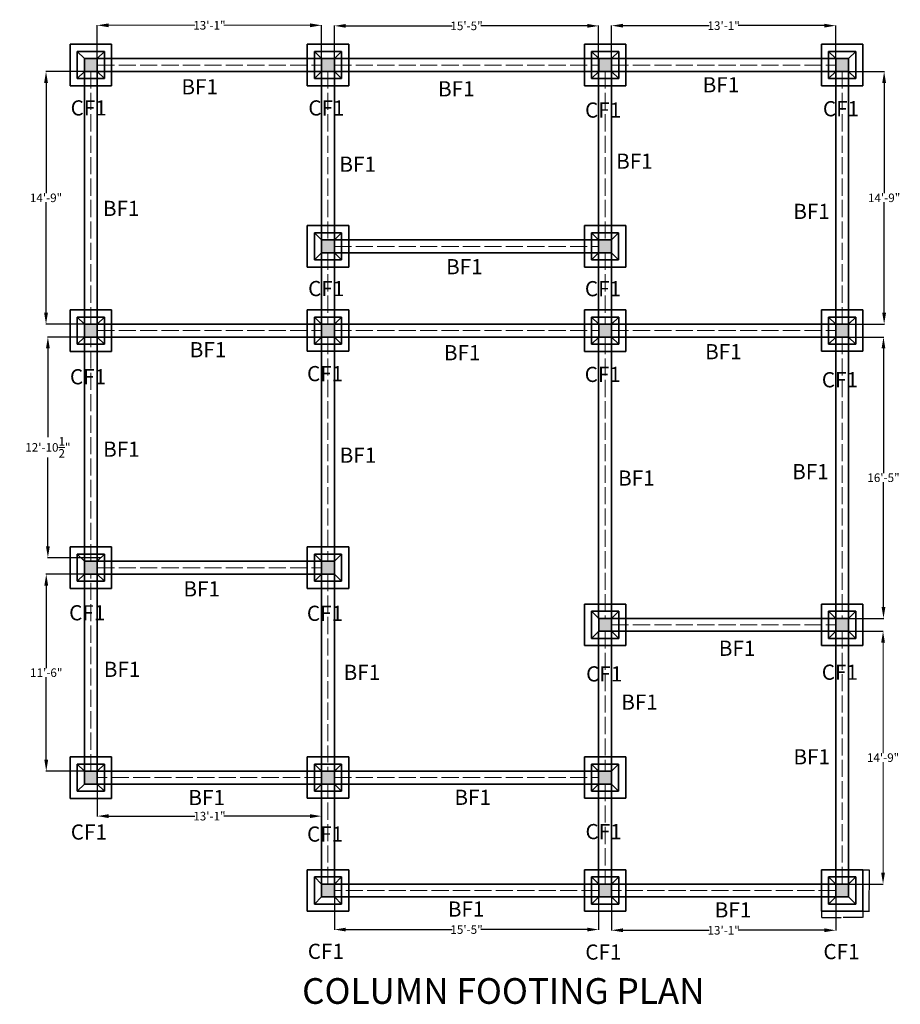
# Model space of a CAD drawing. Units: inches. Extents: x -105 to 1196, y -792 to 119.
# Tile 23 of 23: x 579 to 1196, y -592 to 97. Entities that reach past the tile are written whole.
import ezdxf

# ---------------------------------------------------------------- set-up
doc = ezdxf.new("R2010")
doc.units = ezdxf.units.IN
doc.header["$MEASUREMENT"] = 0
doc.linetypes.add('ACAD_ISO02W100', pattern=[15, 12, -3])
for name, color, linetype, lineweight in [('A-ANNO-DIMS', 2, 'Continuous', 18), ('A-ANNO-TEXT', 7, 'Continuous', 25), ('S-BEAM', 2, 'Continuous', 35), ('S-COLS', 7, 'Continuous', 35), ('S-FNDN', 7, 'Continuous', 35), ('S-GRID', 1, 'ACAD_ISO02W100', 18)]:
    doc.layers.add(name, color=color, linetype=linetype, lineweight=lineweight)
doc.styles.get("Standard").update_dxf_attribs({"font": 'arial.ttf'})
doc.dimstyles.get("Standard").update_dxf_attribs({"dimtxt": 0.18, "dimasz": 0.18, "dimexe": 0.18, "dimexo": 0.0625, "dimgap": 0.09, "dimtad": 0, "dimtih": 1, "dimtoh": 1, "dimdec": 1, "dimzin": 0, "dimdsep": 46, "dimlunit": 4, "dimtxsty": 'Standard', "dimcen": 0.09, "dimadec": 0, "dimazin": 0, "dimtfac": 1, "dimtdec": 1, "dimtofl": 0, "dimtmove": 0, "dimatfit": 3, "dimfxl": 1, "dimtolj": 1, "dimtzin": 0, "dimarcsym": 0})

# ---------------------------------------------------------------- blocks, each defined once
blk = doc.blocks.new('*D40')
at = {"layer": 'A-ANNO-DIMS', "color": 0, "lineweight": -2, "transparency": 16777216}
for p, q in [((799.59, -508.29), (799.59, -540.3)), ((984.59, -508.29), (984.59, -540.3)), ((807.59, -540.12), (881.98, -540.12)), ((976.59, -540.12), (902.21, -540.12))]:
    blk.add_line(p, q, dxfattribs=at)
at = {"layer": 'A-ANNO-DIMS', "color": 0, "transparency": 16777216}
for points in [[(807.59, -538.79), (807.59, -541.46), (799.59, -540.12)], [(976.59, -538.79), (976.59, -541.46), (984.59, -540.12)]]:
    blk.add_solid(points, dxfattribs=at)
at = {"layer": 'Defpoints', "color": 0, "transparency": 16777216}
for p in [(799.59, -508.23), (984.59, -508.23), (984.59, -540.12)]:
    blk.add_point(p, dxfattribs=at)
at = {"layer": 'A-ANNO-DIMS', "color": 0, "transparency": 16777216, "insert": (892.09, -540.12), "char_height": 6, "attachment_point": 5}
blk.add_mtext('\\A1;15\'-5"', dxfattribs=at)
blk = doc.blocks.new('*D41')
at = {"layer": 'A-ANNO-DIMS', "color": 0, "lineweight": -2, "transparency": 16777216}
for p, q in [((993.59, -508.29), (993.59, -540.79)), ((1150.59, -508.29), (1150.59, -540.79)), ((1001.59, -540.61), (1061.98, -540.61)), ((1142.59, -540.61), (1082.21, -540.61))]:
    blk.add_line(p, q, dxfattribs=at)
at = {"layer": 'A-ANNO-DIMS', "color": 0, "transparency": 16777216}
for points in [[(1001.59, -539.27), (1001.59, -541.94), (993.59, -540.61)], [(1142.59, -539.27), (1142.59, -541.94), (1150.59, -540.61)]]:
    blk.add_solid(points, dxfattribs=at)
at = {"layer": 'Defpoints', "color": 0, "transparency": 16777216}
for p in [(993.59, -508.23), (1150.59, -508.23), (1150.59, -540.61)]:
    blk.add_point(p, dxfattribs=at)
at = {"layer": 'A-ANNO-DIMS', "color": 0, "transparency": 16777216, "insert": (1072.09, -540.61), "char_height": 6, "attachment_point": 5}
blk.add_mtext('\\A1;13\'-1"', dxfattribs=at)
blk = doc.blocks.new('*D42')
at = {"layer": 'A-ANNO-DIMS', "color": 0, "lineweight": -2, "transparency": 16777216}
for p, q in [((633.59, -429.29), (633.59, -460.86)), ((790.59, -429.29), (790.59, -460.86)), ((641.59, -460.68), (701.98, -460.68)), ((782.59, -460.68), (722.21, -460.68))]:
    blk.add_line(p, q, dxfattribs=at)
at = {"layer": 'A-ANNO-DIMS', "color": 0, "transparency": 16777216}
for points in [[(641.59, -459.35), (641.59, -462.02), (633.59, -460.68)], [(782.59, -459.35), (782.59, -462.02), (790.59, -460.68)]]:
    blk.add_solid(points, dxfattribs=at)
at = {"layer": 'Defpoints', "color": 0, "transparency": 16777216}
for p in [(633.59, -429.23), (790.59, -429.23), (790.59, -460.68)]:
    blk.add_point(p, dxfattribs=at)
at = {"layer": 'A-ANNO-DIMS', "color": 0, "transparency": 16777216, "insert": (712.09, -460.68), "char_height": 6, "attachment_point": 5}
blk.add_mtext('\\A1;13\'-1"', dxfattribs=at)
blk = doc.blocks.new('*D43')
at = {"layer": 'A-ANNO-DIMS', "color": 0, "lineweight": -2, "transparency": 16777216}
for p, q in [((1150.66, -331.23), (1183.88, -331.23)), ((1150.66, -508.23), (1183.88, -508.23))]:
    blk.add_line(p, q, dxfattribs=at)
at = {"layer": 'A-ANNO-DIMS', "color": 0, "lineweight": 9, "transparency": 16777216}
for p, q in [((1183.7, -339.23), (1183.7, -416.57)), ((1183.7, -500.23), (1183.7, -422.88))]:
    blk.add_line(p, q, dxfattribs=at)
at = {"layer": 'A-ANNO-DIMS', "color": 0, "transparency": 16777216}
for points in [[(1182.36, -339.23), (1185.03, -339.23), (1183.7, -331.23)], [(1182.36, -500.23), (1185.03, -500.23), (1183.7, -508.23)]]:
    blk.add_solid(points, dxfattribs=at)
at = {"layer": 'Defpoints', "color": 0, "transparency": 16777216}
for p in [(1150.59, -331.23), (1183.7, -331.23), (1150.59, -508.23)]:
    blk.add_point(p, dxfattribs=at)
at = {"layer": 'A-ANNO-DIMS', "color": 0, "transparency": 16777216, "insert": (1183.7, -419.73), "char_height": 6, "attachment_point": 5}
blk.add_mtext('\\A1;14\'-9"', dxfattribs=at)
blk = doc.blocks.new('*D44')
at = {"layer": 'A-ANNO-DIMS', "color": 0, "lineweight": -2, "transparency": 16777216}
for p, q in [((1150.66, -125.23), (1184.17, -125.23)), ((1183.99, -133.23), (1183.99, -220.57)), ((1183.99, -314.23), (1183.99, -226.88)), ((1150.66, -322.23), (1184.17, -322.23))]:
    blk.add_line(p, q, dxfattribs=at)
at = {"layer": 'A-ANNO-DIMS', "color": 0, "transparency": 16777216}
for points in [[(1182.66, -133.23), (1185.32, -133.23), (1183.99, -125.23)], [(1182.66, -314.23), (1185.32, -314.23), (1183.99, -322.23)]]:
    blk.add_solid(points, dxfattribs=at)
at = {"layer": 'Defpoints', "color": 0, "transparency": 16777216}
for p in [(1150.59, -125.23), (1183.99, -125.23), (1150.59, -322.23)]:
    blk.add_point(p, dxfattribs=at)
at = {"layer": 'A-ANNO-DIMS', "color": 0, "transparency": 16777216, "insert": (1183.99, -223.73), "char_height": 6, "attachment_point": 5}
blk.add_mtext('\\A1;16\'-5"', dxfattribs=at)
blk = doc.blocks.new('*D45')
at = {"layer": 'A-ANNO-DIMS', "color": 0, "lineweight": -2, "transparency": 16777216}
for p, q in [((1150.66, 60.77), (1184.63, 60.77)), ((1184.45, 52.77), (1184.45, -24.57)), ((1184.45, -108.23), (1184.45, -30.88)), ((1150.66, -116.23), (1184.63, -116.23))]:
    blk.add_line(p, q, dxfattribs=at)
at = {"layer": 'A-ANNO-DIMS', "color": 0, "transparency": 16777216}
for points in [[(1183.12, 52.77), (1185.79, 52.77), (1184.45, 60.77)], [(1183.12, -108.23), (1185.79, -108.23), (1184.45, -116.23)]]:
    blk.add_solid(points, dxfattribs=at)
at = {"layer": 'Defpoints', "color": 0, "transparency": 16777216}
for p in [(1150.59, 60.77), (1184.45, 60.77), (1150.59, -116.23)]:
    blk.add_point(p, dxfattribs=at)
at = {"layer": 'A-ANNO-DIMS', "color": 0, "transparency": 16777216, "insert": (1184.45, -27.73), "char_height": 6, "attachment_point": 5}
blk.add_mtext('\\A1;14\'-9"', dxfattribs=at)
blk = doc.blocks.new('*D46')
at = {"layer": 'A-ANNO-DIMS', "color": 0, "lineweight": -2, "transparency": 16777216}
for p, q in [((993.59, 60.84), (993.59, 93)), ((1001.59, 92.82), (1061.98, 92.82)), ((1142.59, 92.82), (1082.21, 92.82)), ((1150.59, 60.84), (1150.59, 93))]:
    blk.add_line(p, q, dxfattribs=at)
at = {"layer": 'A-ANNO-DIMS', "color": 0, "transparency": 16777216}
for points in [[(1001.59, 94.15), (1001.59, 91.49), (993.59, 92.82)], [(1142.59, 94.15), (1142.59, 91.49), (1150.59, 92.82)]]:
    blk.add_solid(points, dxfattribs=at)
at = {"layer": 'Defpoints', "color": 0, "transparency": 16777216}
for p in [(1150.59, 92.82), (993.59, 60.77), (1150.59, 60.77)]:
    blk.add_point(p, dxfattribs=at)
at = {"layer": 'A-ANNO-DIMS', "color": 0, "transparency": 16777216, "insert": (1072.09, 92.82), "char_height": 6, "attachment_point": 5}
blk.add_mtext('\\A1;13\'-1"', dxfattribs=at)
blk = doc.blocks.new('*D47')
at = {"layer": 'A-ANNO-DIMS', "color": 0, "lineweight": -2, "transparency": 16777216}
for p, q in [((799.59, 60.84), (799.59, 92.86)), ((807.59, 92.68), (881.98, 92.68)), ((976.59, 92.68), (902.21, 92.68)), ((984.59, 60.84), (984.59, 92.86))]:
    blk.add_line(p, q, dxfattribs=at)
at = {"layer": 'A-ANNO-DIMS', "color": 0, "transparency": 16777216}
for points in [[(807.59, 94.02), (807.59, 91.35), (799.59, 92.68)], [(976.59, 94.02), (976.59, 91.35), (984.59, 92.68)]]:
    blk.add_solid(points, dxfattribs=at)
at = {"layer": 'Defpoints', "color": 0, "transparency": 16777216}
for p in [(984.59, 92.68), (799.59, 60.77), (984.59, 60.77)]:
    blk.add_point(p, dxfattribs=at)
at = {"layer": 'A-ANNO-DIMS', "color": 0, "transparency": 16777216, "insert": (892.09, 92.68), "char_height": 6, "attachment_point": 5}
blk.add_mtext('\\A1;15\'-5"', dxfattribs=at)
blk = doc.blocks.new('*D48')
at = {"layer": 'A-ANNO-DIMS', "color": 0, "lineweight": -2, "transparency": 16777216}
for p, q in [((633.59, 60.84), (633.59, 93.25)), ((790.59, 60.84), (790.59, 93.25))]:
    blk.add_line(p, q, dxfattribs=at)
at = {"layer": 'A-ANNO-DIMS', "color": 0, "lineweight": 5, "transparency": 16777216}
for p, q in [((641.59, 93.07), (701.98, 93.07)), ((782.59, 93.07), (722.21, 93.07))]:
    blk.add_line(p, q, dxfattribs=at)
at = {"layer": 'A-ANNO-DIMS', "color": 0, "transparency": 16777216}
for points in [[(641.59, 94.4), (641.59, 91.73), (633.59, 93.07)], [(782.59, 94.4), (782.59, 91.73), (790.59, 93.07)]]:
    blk.add_solid(points, dxfattribs=at)
at = {"layer": 'Defpoints', "color": 0, "transparency": 16777216}
for p in [(790.59, 93.07), (633.59, 60.77), (790.59, 60.77)]:
    blk.add_point(p, dxfattribs=at)
at = {"layer": 'A-ANNO-DIMS', "color": 0, "transparency": 16777216, "insert": (712.09, 93.07), "char_height": 6, "attachment_point": 5}
blk.add_mtext('\\A1;13\'-1"', dxfattribs=at)
blk = doc.blocks.new('*D49')
at = {"layer": 'A-ANNO-DIMS', "color": 0, "lineweight": -2, "transparency": 16777216}
for p, q in [((633.53, 60.77), (597.53, 60.77)), ((597.71, 52.77), (597.71, -24.57)), ((597.71, -108.23), (597.71, -30.88)), ((633.53, -116.23), (597.53, -116.23))]:
    blk.add_line(p, q, dxfattribs=at)
at = {"layer": 'A-ANNO-DIMS', "color": 0, "transparency": 16777216}
for points in [[(596.38, 52.77), (599.04, 52.77), (597.71, 60.77)], [(596.38, -108.23), (599.04, -108.23), (597.71, -116.23)]]:
    blk.add_solid(points, dxfattribs=at)
at = {"layer": 'Defpoints', "color": 0, "transparency": 16777216}
for p in [(633.59, 60.77), (597.71, -116.23), (633.59, -116.23)]:
    blk.add_point(p, dxfattribs=at)
at = {"layer": 'A-ANNO-DIMS', "color": 0, "transparency": 16777216, "insert": (597.71, -27.73), "char_height": 6, "attachment_point": 5}
blk.add_mtext('\\A1;14\'-9"', dxfattribs=at)
blk = doc.blocks.new('*D50')
at = {"layer": 'A-ANNO-DIMS', "color": 0, "lineweight": -2, "transparency": 16777216}
for p, q in [((633.53, -125.23), (598.82, -125.23)), ((599, -133.23), (599, -195.31)), ((599, -271.73), (599, -209.64)), ((636.03, -279.73), (598.82, -279.73))]:
    blk.add_line(p, q, dxfattribs=at)
at = {"layer": 'A-ANNO-DIMS', "color": 0, "transparency": 16777216}
for points in [[(597.67, -133.23), (600.33, -133.23), (599, -125.23)], [(597.67, -271.73), (600.33, -271.73), (599, -279.73)]]:
    blk.add_solid(points, dxfattribs=at)
at = {"layer": 'Defpoints', "color": 0, "transparency": 16777216}
for p in [(633.59, -125.23), (599, -279.73), (636.09, -279.73)]:
    blk.add_point(p, dxfattribs=at)
at = {"layer": 'A-ANNO-DIMS', "color": 0, "transparency": 16777216, "insert": (599, -202.48), "char_height": 6, "attachment_point": 5}
blk.add_mtext('\\A1;12\'-10{\\H1x;\\S1/2;}"', dxfattribs=at)
blk = doc.blocks.new('*D51')
at = {"layer": 'A-ANNO-DIMS', "color": 0, "lineweight": -2, "transparency": 16777216}
for p, q in [((633.53, -291.23), (597.67, -291.23)), ((597.85, -299.23), (597.85, -357.07)), ((597.85, -421.23), (597.85, -363.38)), ((633.53, -429.23), (597.67, -429.23))]:
    blk.add_line(p, q, dxfattribs=at)
at = {"layer": 'A-ANNO-DIMS', "color": 0, "transparency": 16777216}
for points in [[(596.51, -299.23), (599.18, -299.23), (597.85, -291.23)], [(596.51, -421.23), (599.18, -421.23), (597.85, -429.23)]]:
    blk.add_solid(points, dxfattribs=at)
at = {"layer": 'Defpoints', "color": 0, "transparency": 16777216}
for p in [(633.59, -291.23), (597.85, -429.23), (633.59, -429.23)]:
    blk.add_point(p, dxfattribs=at)
at = {"layer": 'A-ANNO-DIMS', "color": 0, "transparency": 16777216, "insert": (597.85, -360.23), "char_height": 6, "attachment_point": 5}
blk.add_mtext('\\A1;11\'-6"', dxfattribs=at)
blk = doc.blocks.new('FTG-CF1')
at = {"ltscale": 0.5}
for p, q in [((614.59, 79.77), (643.59, 79.77)), ((614.59, 50.77), (614.59, 79.77)), ((643.59, 79.77), (643.59, 50.77)), ((643.59, 50.77), (614.59, 50.77))]:
    blk.add_line(p, q, dxfattribs=at)
for p, q in [((624.59, 69.77), (619.59, 74.77)), ((619.59, 55.77), (619.59, 74.77)), ((619.59, 74.77), (638.59, 74.77)), ((624.59, 60.77), (624.59, 69.77)), ((624.59, 69.77), (633.59, 69.77)), ((633.59, 69.77), (638.59, 74.77)), ((633.59, 69.77), (633.59, 60.77)), ((638.59, 74.77), (638.59, 55.77)), ((619.59, 55.77), (624.59, 60.77)), ((638.59, 55.77), (619.59, 55.77)), ((633.59, 60.77), (624.59, 60.77)), ((633.59, 60.77), (638.59, 55.77))]:
    blk.add_line(p, q)
blk = doc.blocks.new('*D89')
at = {"layer": 'A-ANNO-DIMS', "color": 0, "lineweight": -2, "transparency": 16777216}
for p, q in [((1169.66, -498.23), (1174.12, -498.23)), ((1173.94, -498.41), (1173.94, -512.54)), ((1173.94, -527.05), (1173.94, -512.91)), ((1169.66, -527.23), (1174.12, -527.23))]:
    blk.add_line(p, q, dxfattribs=at)
at = {"layer": 'A-ANNO-DIMS', "color": 0, "transparency": 16777216}
for points in [[(1173.91, -498.41), (1173.97, -498.41), (1173.94, -498.23)], [(1173.91, -527.05), (1173.97, -527.05), (1173.94, -527.23)]]:
    blk.add_solid(points, dxfattribs=at)
at = {"layer": 'Defpoints', "color": 0, "transparency": 16777216}
for p in [(1169.59, -498.23), (1169.59, -527.23), (1173.94, -527.23)]:
    blk.add_point(p, dxfattribs=at)
at = {"layer": 'A-ANNO-DIMS', "color": 0, "transparency": 16777216, "insert": (1173.94, -512.73), "char_height": 0.18, "attachment_point": 5}
blk.add_mtext('\\A1;FOOTING CF1 2\'-5" TYP.', dxfattribs=at)
blk = doc.blocks.new('*D90')
at = {"layer": 'A-ANNO-DIMS', "color": 0, "lineweight": -2, "transparency": 16777216}
for p, q in [((1140.59, -527.29), (1140.59, -531.76)), ((1169.59, -527.29), (1169.59, -531.76)), ((1140.77, -531.58), (1154.45, -531.58)), ((1169.41, -531.58), (1155.74, -531.58))]:
    blk.add_line(p, q, dxfattribs=at)
at = {"layer": 'A-ANNO-DIMS', "color": 0, "transparency": 16777216}
for points in [[(1140.77, -531.55), (1140.77, -531.61), (1140.59, -531.58)], [(1169.41, -531.55), (1169.41, -531.61), (1169.59, -531.58)]]:
    blk.add_solid(points, dxfattribs=at)
at = {"layer": 'Defpoints', "color": 0, "transparency": 16777216}
for p in [(1140.59, -527.23), (1169.59, -527.23), (1140.59, -531.58)]:
    blk.add_point(p, dxfattribs=at)
at = {"layer": 'A-ANNO-DIMS', "color": 0, "transparency": 16777216, "insert": (1155.09, -531.58), "char_height": 0.18, "attachment_point": 5}
blk.add_mtext('\\A1;2\'-5" TYP.', dxfattribs=at)

msp = doc.modelspace()

# ---------------------------------------------------------------- hatches: boundary and pattern name
at = {"layer": 'S-COLS'}
h = msp.add_hatch(color=256, dxfattribs=at)
h.dxf.hatch_style = 1
h.paths.add_polyline_path([(633.59, 69.77), (624.59, 69.77), (624.59, 60.77), (633.59, 60.77)])
h.paths.add_polyline_path([(799.59, 69.77), (790.59, 69.77), (790.59, 60.77), (799.59, 60.77)])
h.paths.add_polyline_path([(993.59, 69.77), (984.59, 69.77), (984.59, 60.77), (993.59, 60.77)])
h.paths.add_polyline_path([(1159.59, 69.77), (1150.59, 69.77), (1150.59, 60.77), (1159.59, 60.77)])
h.paths.add_polyline_path([(799.59, -57.23), (790.59, -57.23), (790.59, -66.23), (799.59, -66.23)])
h.paths.add_polyline_path([(993.59, -57.23), (984.59, -57.23), (984.59, -66.23), (993.59, -66.23)])
h.paths.add_polyline_path([(993.59, -116.23), (984.59, -116.23), (984.59, -125.23), (993.59, -125.23)])
h.paths.add_polyline_path([(1159.59, -116.23), (1150.59, -116.23), (1150.59, -125.23), (1159.59, -125.23)])
h.paths.add_polyline_path([(799.59, -116.23), (790.59, -116.23), (790.59, -125.23), (799.59, -125.23)])
h.paths.add_polyline_path([(633.59, -116.23), (624.59, -116.23), (624.59, -125.23), (633.59, -125.23)])
h.paths.add_polyline_path([(633.59, -282.23), (624.59, -282.23), (624.59, -291.23), (633.59, -291.23)])
h.paths.add_polyline_path([(799.59, -282.23), (790.59, -282.23), (790.59, -291.23), (799.59, -291.23)])
h.paths.add_polyline_path([(633.59, -429.23), (624.59, -429.23), (624.59, -438.23), (633.59, -438.23)])
h.paths.add_polyline_path([(799.59, -429.23), (790.59, -429.23), (790.59, -438.23), (799.59, -438.23)])
h.paths.add_polyline_path([(799.59, -508.23), (790.59, -508.23), (790.59, -517.23), (799.59, -517.23)])
h.paths.add_polyline_path([(993.59, -429.23), (984.59, -429.23), (984.59, -438.23), (993.59, -438.23)])
h.paths.add_polyline_path([(993.59, -508.23), (984.59, -508.23), (984.59, -517.23), (993.59, -517.23)])
h.paths.add_polyline_path([(993.59, -322.23), (984.59, -322.23), (984.59, -331.23), (993.59, -331.23)])
h.paths.add_polyline_path([(1159.59, -322.23), (1150.59, -322.23), (1150.59, -331.23), (1159.59, -331.23)])
h.paths.add_polyline_path([(1159.59, -508.23), (1150.59, -508.23), (1150.59, -517.23), (1159.59, -517.23)])

# ---------------------------------------------------------------- linework, layer by layer
at = {"layer": 'S-BEAM'}
for p, q in [((633.59, 69.77), (790.59, 69.77)), ((799.59, 69.77), (984.59, 69.77)), ((993.59, 69.77), (1150.59, 69.77)), ((624.59, 60.77), (624.59, -116.23)), ((633.59, 60.77), (790.59, 60.77)), ((633.59, 60.77), (633.59, -116.23)), ((790.59, 60.77), (790.59, -57.23)), ((799.59, 60.77), (984.59, 60.77)), ((799.59, 60.77), (799.59, -57.23)), ((984.59, 60.77), (984.59, -57.23)), ((993.59, 60.77), (1150.59, 60.77)), ((993.59, 60.77), (993.59, -57.23)), ((1150.59, 60.77), (1150.59, -116.23)), ((1159.59, 60.77), (1159.59, -116.23)), ((799.59, -57.23), (984.59, -57.23)), ((790.59, -66.23), (790.59, -116.23)), ((799.59, -66.23), (984.59, -66.23)), ((799.59, -66.23), (799.59, -116.23)), ((984.59, -66.23), (984.59, -116.23)), ((993.59, -66.23), (993.59, -116.23)), ((633.59, -116.23), (790.59, -116.23)), ((799.59, -116.23), (984.59, -116.23)), ((993.59, -116.23), (1150.59, -116.23)), ((624.59, -125.23), (624.59, -282.23)), ((633.59, -125.23), (790.59, -125.23)), ((633.59, -125.23), (633.59, -282.23)), ((790.59, -125.23), (790.59, -282.23)), ((799.59, -125.23), (984.59, -125.23)), ((799.59, -125.23), (799.59, -282.23)), ((984.59, -125.23), (984.59, -322.23)), ((993.59, -125.23), (1150.59, -125.23)), ((993.59, -125.23), (993.59, -322.23)), ((1150.59, -125.23), (1150.59, -322.23)), ((1159.59, -125.23), (1159.59, -322.23)), ((633.59, -282.23), (790.59, -282.23)), ((624.59, -291.23), (624.59, -429.23)), ((633.59, -291.23), (790.59, -291.23)), ((633.59, -291.23), (633.59, -429.23)), ((790.59, -291.23), (790.59, -429.23)), ((799.59, -291.23), (799.59, -429.23)), ((993.59, -322.23), (1150.59, -322.23)), ((984.59, -331.23), (984.59, -429.23)), ((993.59, -331.23), (1150.59, -331.23)), ((993.59, -331.23), (993.59, -429.23)), ((1150.59, -331.23), (1150.59, -508.23)), ((1159.59, -331.23), (1159.59, -508.23)), ((633.59, -429.23), (790.59, -429.23)), ((799.59, -429.23), (984.59, -429.23)), ((633.59, -438.23), (790.59, -438.23)), ((790.59, -438.23), (790.59, -508.23)), ((799.59, -438.23), (984.59, -438.23)), ((799.59, -438.23), (799.59, -508.23)), ((984.59, -438.23), (984.59, -508.23)), ((993.59, -438.23), (993.59, -508.23)), ((799.59, -508.23), (984.59, -508.23)), ((993.59, -508.23), (1150.59, -508.23)), ((799.59, -517.23), (984.59, -517.23)), ((993.59, -517.23), (1150.59, -517.23))]:
    msp.add_line(p, q, dxfattribs=at)
at = {"layer": 'S-FNDN'}
for p, q in [((799.59, -282.23), (799.59, -291.23)), ((1150.59, -517.23), (1150.59, -508.23))]:
    msp.add_line(p, q, dxfattribs=at)
at = {"layer": 'S-GRID'}
for p, q in [((633.59, 65.27), (790.59, 65.27)), ((799.59, 65.27), (984.59, 65.27)), ((993.59, 65.27), (1150.59, 65.27)), ((629.09, -116.23), (629.09, 60.77)), ((795.09, 60.77), (795.09, -57.23)), ((989.09, 60.77), (989.09, -57.23)), ((1155.09, 60.77), (1155.09, -116.23)), ((799.59, -61.73), (984.59, -61.73)), ((795.09, -66.23), (795.09, -116.23)), ((989.09, -66.23), (989.09, -116.23)), ((633.59, -120.73), (790.59, -120.73)), ((799.59, -120.73), (984.59, -120.73)), ((993.59, -120.73), (1150.59, -120.73)), ((629.09, -282.23), (629.09, -125.23)), ((795.09, -125.23), (795.09, -282.23)), ((989.09, -125.23), (989.09, -322.23)), ((1155.09, -125.23), (1155.09, -322.23)), ((633.59, -286.73), (790.59, -286.73)), ((629.09, -429.23), (629.09, -291.23)), ((795.09, -291.23), (795.09, -429.23)), ((993.59, -326.73), (1150.59, -326.73)), ((989.09, -331.23), (989.09, -429.23)), ((1155.09, -331.23), (1155.09, -508.23)), ((790.59, -433.73), (633.59, -433.73)), ((799.59, -433.73), (984.6, -433.73)), ((795.09, -508.23), (795.09, -438.23)), ((989.09, -438.23), (989.09, -508.23)), ((984.59, -512.73), (799.59, -512.73)), ((1150.59, -512.73), (993.59, -512.73))]:
    msp.add_line(p, q, dxfattribs=at)

# ---------------------------------------------------------------- block references
at = {"layer": 'S-FNDN'}
for p, rotation in [((563.82, 694.37), 270.0000000000001), ((1618.19, 130.55), 180), ((1089.82, 694.37), 269.9999999999985), ((1424.19, 3.55), 180), ((923.82, 567.37), 269.9999999999992), ((694.37, -749.82), 89.9999999999995), ((729.82, 508.37), 269.9999999999994), ((1054.37, -749.82), 90.00000000000081), ((1089.82, 508.37), 269.9999999999985), ((694.37, -915.82), 89.9999999999995), ((729.82, 342.37), 269.9999999999995), ((1054.37, -955.82), 90.00000000000072), ((1089.82, 302.37), 270), ((694.37, -1062.82), 89.9999999999996), ((1424.19, -368.45), 180), ((923.82, 195.37), 269.9999999999993), ((1424.19, -447.45), 180), ((1618.19, -447.45), 180), ((1784.19, -447.45), 180)]:
    msp.add_blockref('FTG-CF1', p, dxfattribs=dict(at, rotation=rotation))
msp.add_blockref('FTG-CF1', (166, 0), dxfattribs=at)

# ---------------------------------------------------------------- texts
at = {"layer": 'A-ANNO-TEXT'}
for s, height, p in [('BF1', 10.636, (692.48, 44.7)), ('BF1', 10.636, (1057.43, 46.11)), ('BF1', 10.636, (872.14, 43.29)), ('CF1', 10.636, (614.91, 29.92)), ('CF1', 10.636, (781.31, 29.89)), ('CF1', 10.636, (975.05, 28.41)), ('CF1', 10.636, (1141.56, 29.34)), ('BF1', 10.636, (803.09, -9.49)), ('BF1', 10.636, (996.84, -7.38)), ('BF1', 10.636, (637.53, -40.46)), ('BF1', 10.636, (1120.84, -42.57)), ('BF1', 10.636, (877.77, -81.27)), ('CF1', 10.636, (781.16, -96.58)), ('CF1', 10.636, (974.93, -96.67)), ('BF1', 10.636, (698.31, -139.39)), ('BF1', 10.636, (876.26, -141.49)), ('BF1', 10.636, (1059.12, -140.79)), ('CF1', 10.636, (614.42, -158.33)), ('CF1', 10.636, (780.41, -156.14)), ('CF1', 10.636, (974.79, -156.69)), ('CF1', 10.636, (1140.82, -160.43)), ('BF1', 10.636, (637.7, -209.05)), ('BF1', 10.636, (803.28, -213.24)), ('BF1', 10.636, (998.2, -229.29)), ('BF1', 10.636, (1120.07, -224.77)), ('BF1', 10.636, (693.88, -306.84)), ('CF1', 10.636, (613.85, -323.6)), ('CF1', 10.636, (780.32, -323.97)), ('BF1', 10.636, (1068.7, -348.44)), ('BF1', 10.636, (638.15, -363.21)), ('BF1', 10.636, (806.05, -365.3)), ('CF1', 10.636, (975.79, -366.4)), ('CF1', 10.636, (1140.75, -365.21)), ('BF1', 10.636, (1000.42, -386.18)), ('BF1', 10.636, (1120.95, -424.45)), ('BF1', 10.636, (697.37, -452.99)), ('BF1', 10.636, (883.61, -452.82)), ('CF1', 10.636, (615.03, -477.13)), ('CF1', 10.636, (780.41, -478.55)), ('CF1', 10.636, (975.36, -476.83)), ('BF1', 10.636, (879.03, -531.09)), ('BF1', 10.636, (1065.85, -531.65)), ('CF1', 10.636, (780.93, -560.67)), ('CF1', 10.636, (975.23, -561.18)), ('CF1', 10.636, (1141.9, -560.88)), ('COLUMN FOOTING PLAN', 18, (776.96, -592.13))]:
    msp.add_text(s, height=height, dxfattribs=at).set_placement(p)

# ---------------------------------------------------------------- dimensions: what is measured, and where the dimension line sits
at = {"layer": 'A-ANNO-DIMS'}
for base, p1, p2, override, picture, middle in [((790.59, 93.07), (633.59, 60.77), (790.59, 60.77), {"dimtxt": 6, "dimasz": 8, "dimclrd": 0, "dimclre": 0, "dimclrt": 0, "dimlwd": 5}, '*D48', (712.09, 93.07)), ((984.59, 92.68), (799.59, 60.77), (984.59, 60.77), {"dimtxt": 6, "dimasz": 8, "dimclrd": 0, "dimclre": 0, "dimclrt": 0}, '*D47', (892.09, 92.68)), ((1150.59, 92.82), (993.59, 60.77), (1150.59, 60.77), {"dimtxt": 6, "dimasz": 8, "dimclrd": 0, "dimclre": 0, "dimclrt": 0}, '*D46', (1072.09, 92.82)), ((790.59, -460.68), (633.59, -429.23), (790.59, -429.23), {"dimtxt": 6, "dimasz": 8, "dimclrd": 0, "dimclre": 0, "dimclrt": 0}, '*D42', (712.09, -460.68)), ((984.59, -540.12), (799.59, -508.23), (984.59, -508.23), {"dimtxt": 6, "dimasz": 8, "dimclrd": 0, "dimclre": 0, "dimclrt": 0}, '*D40', (892.09, -540.12)), ((1150.59, -540.61), (993.59, -508.23), (1150.59, -508.23), {"dimtxt": 6, "dimasz": 8, "dimclrd": 0, "dimclre": 0, "dimclrt": 0}, '*D41', (1072.09, -540.61))]:
    dim = msp.add_linear_dim(base=base, p1=p1, p2=p2, dimstyle='Standard', override=override, dxfattribs=at)
    dim.commit()
    dim.dimension.update_dxf_attribs({"geometry": picture, "text_midpoint": middle})
for base, p1, p2, override, picture, middle in [((597.71, -116.23), (633.59, 60.77), (633.59, -116.23), {"dimtxt": 6, "dimasz": 8, "dimclrd": 0, "dimclre": 0, "dimclrt": 0}, '*D49', (597.71, -27.73)), ((1184.45, 60.77), (1150.59, -116.23), (1150.59, 60.77), {"dimtxt": 6, "dimasz": 8, "dimclrd": 0, "dimclre": 0, "dimclrt": 0}, '*D45', (1184.45, -27.73)), ((599, -279.73), (633.59, -125.23), (636.09, -279.73), {"dimtxt": 6, "dimasz": 8, "dimclrd": 0, "dimclre": 0, "dimclrt": 0}, '*D50', (599, -202.48)), ((1183.99, -125.23), (1150.59, -322.23), (1150.59, -125.23), {"dimtxt": 6, "dimasz": 8, "dimclrd": 0, "dimclre": 0, "dimclrt": 0}, '*D44', (1183.99, -223.73)), ((597.85, -429.23), (633.59, -291.23), (633.59, -429.23), {"dimtxt": 6, "dimasz": 8, "dimclrd": 0, "dimclre": 0, "dimclrt": 0}, '*D51', (597.85, -360.23)), ((1183.7, -331.23), (1150.59, -508.23), (1150.59, -331.23), {"dimtxt": 6, "dimasz": 8, "dimclrd": 0, "dimclre": 0, "dimclrt": 0, "dimlwd": 9}, '*D43', (1183.7, -419.73))]:
    dim = msp.add_linear_dim(base=base, p1=p1, p2=p2, angle=90, dimstyle='Standard', override=override, dxfattribs=at)
    dim.commit()
    dim.dimension.update_dxf_attribs({"geometry": picture, "text_midpoint": middle})
for base, p1, p2, angle, text, picture, middle in [((1173.94, -527.23), (1169.59, -498.23), (1169.59, -527.23), 270, 'FOOTING CF1 <> TYP.', '*D89', (1173.94, -512.73)), ((1140.59, -531.58), (1169.59, -527.23), (1140.59, -527.23), 180, '<> TYP.', '*D90', (1155.09, -531.58))]:
    dim = msp.add_linear_dim(base=base, p1=p1, p2=p2, angle=angle, text=text, dimstyle='Standard', override={"dimdec": 1, "dimlfac": 1, "dimrnd": 0, "dimzin": 1, "dimdsep": 46, "dimlunit": 4, "dimfrac": 2}, dxfattribs=at)
    dim.commit()
    dim.dimension.update_dxf_attribs({"geometry": picture, "text_midpoint": middle})

doc.saveas('drawing.dxf')
